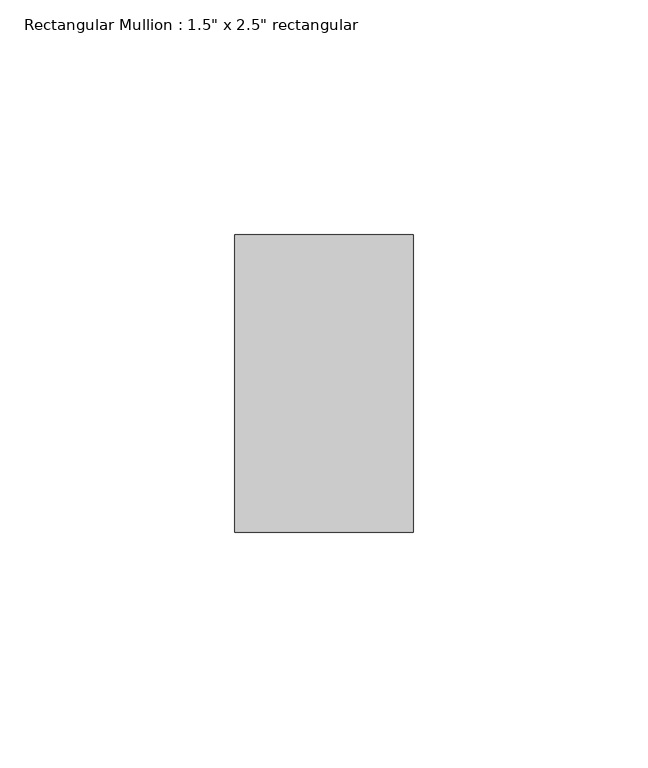
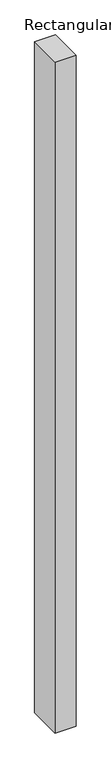
"""IFC4 building model written with IfcOpenShell, lengths in millimetres: member geometry."""

from ifc_helpers import new_model, si_unit, frame, origin, place, context, project, spatial, polyline, outline, extrude, source, transform, mapped, element, save


def member_9069d910(model_context):
    return source(origin(), model_context, "Body", "SweptSolid", [
        extrude(outline(polyline([(0.0, 31.75), (0.0, -31.75), (-38.1, -31.75), (-38.1, 31.75), (0.0, 31.75)])), frame((0.0, 0.0, -1282.7), z_axis=(0.0, 0.0, 1.0), x_axis=(1.0, 0.0, 0.0)), (0.0, 0.0, 1.0), 1282.7),
    ])


if __name__ == "__main__":
    model = new_model("IFC4")
    model_context = context("Model", 3, world=origin())
    ifc_project = project(units=[si_unit("LENGTHUNIT", "METRE", prefix="MILLI")], contexts=[model_context])
    site = spatial("IfcSite", under=ifc_project)
    building = spatial("IfcBuilding", under=site)
    placement = place(None, origin())
    member_shape = member_9069d910(model_context)
    element("IfcMember", 1, ObjectType="Rectangular Mullion : 1.5\" x 2.5\" rectangular", at=placement, inside=building, context=model_context, shape_type="MappedRepresentation", body=[
        mapped(member_shape, transform((0.0, 0.0, 0.0), x_axis=(1.0, 0.0, 0.0), y_axis=(0.0, 1.0, 0.0), z_axis=(0.0, 0.0, 1.0))),
    ])
    save(model, "model.ifc")

# Revit data of these elements
# Type "Rectangular Mullion : 1.5\" x 2.5\" rectangular"
#   built-in parameter 1007304 = 0.208333 (stored number, unit not read)
#   built-in parameter 1007301 = 0.0625 (stored number, unit not read)
#   built-in parameter 1007300 = 0.0625 (stored number, unit not read)
# Element 1 (IfcMember, "Rectangular Mullion : 1.5\" x 2.5\" rectangular")
#   Materials on its faces: "Damp-proofing"
# Materials
#   "Damp-proofing": class "Generic", colour RGB 127 127 127, transparency 0, Description = "Damp-proofing", Cost = 0
